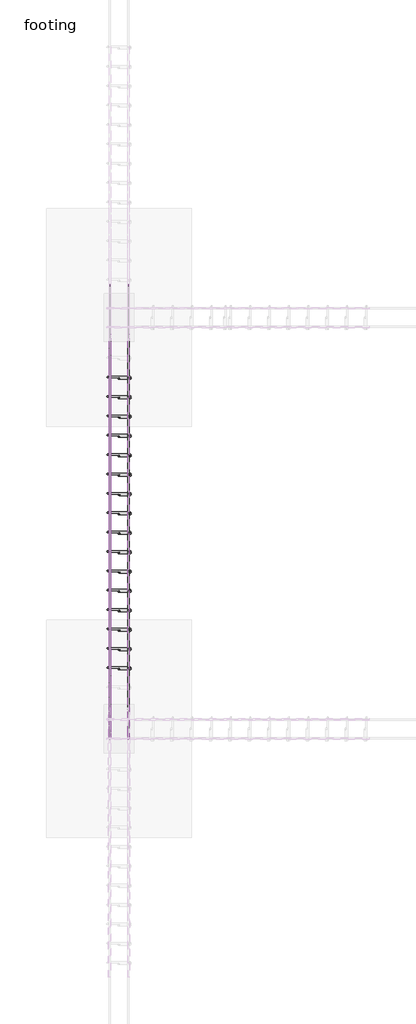
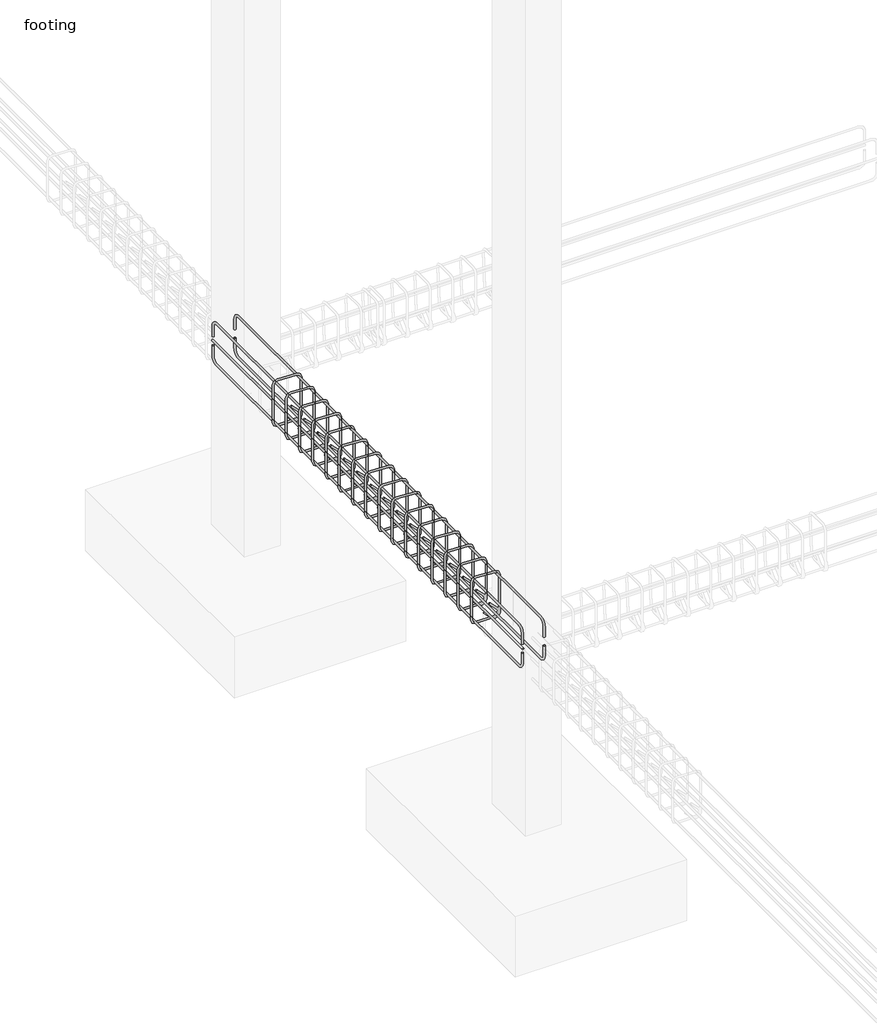
# One storey, part 5 of 21: 22 reinforcing bars.
"""IFC4 building model written with IfcOpenShell, lengths in millimetres."""

from ifc_helpers import new_model, si_unit, point, frame, origin, place, context, project, spatial, polyline, circle_curve, trimmed, segment, composite_curve, element, save
from ifc_brep_helpers import swept_disk

model = new_model("IFC4")

# Units and contexts
model_context = context("Model", 3, world=origin())
ifc_project = project(units=[si_unit("LENGTHUNIT", "METRE", prefix="MILLI")], contexts=[model_context])

# Site, building, storey
site = spatial("IfcSite", under=ifc_project)
building = spatial("IfcBuilding", under=site)
storey = spatial("IfcBuildingStorey", under=building, Name="footing", Elevation=-1524.0)

# Reinforcing bars
placement = place(None, origin())
element("IfcReinforcingBar", 1, at=placement, inside=storey, context=model_context, shape_type="SolidModel", body=[
    swept_disk(composite_curve([segment(polyline([(-12178.1165254, 4620.1956073, -265.9812362), (-12123.251527, 4620.1956073, -320.8462347)]), True, "CONTINUOUS"), segment(trimmed(circle_curve(frame((-12145.7021673, 4620.1956073, -343.296875), z_axis=(0.0, 1.0, 0.0), x_axis=(22.450640299999577, 0.0, 22.450640299999975)), 31.75), [point((-12123.251527, 4620.1956073, -320.8462347))], [point((-12145.7021673, 4620.1956073, -375.046875))], True, "CARTESIAN"), True, "CONTINUOUS"), segment(polyline([(-12145.7021673, 4620.1956073, -375.046875), (-12273.4959173, 4620.1956073, -375.046875)]), True, "CONTINUOUS"), segment(trimmed(circle_curve(frame((-12273.4959173, 4620.1956073, -343.296875), z_axis=(0.0, 1.0, 0.0), x_axis=(0.0, 0.0, -31.75)), 31.75), [point((-12273.4959173, 4620.1956073, -375.046875))], [point((-12305.2459173, 4620.1956073, -343.296875))], True, "CARTESIAN"), True, "CONTINUOUS"), segment(polyline([(-12305.2459173, 4620.1956073, -343.296875), (-12305.2459173, 4620.1956073, -63.103125)]), True, "CONTINUOUS"), segment(trimmed(circle_curve(frame((-12273.565658, 4618.0923536, -63.103125), z_axis=(0.0662442117686417, 0.9978034397651431, 0.0), x_axis=(-31.680259300001126, 2.1032537000000957, 0.0)), 31.75), [point((-12305.2459173, 4620.1956073, -63.103125))], [point((-12273.565658, 4618.0923536, -31.353125))], True, "CARTESIAN"), True, "CONTINUOUS"), segment(polyline([(-12273.565658, 4618.0923536, -31.353125), (-12145.6324265, 4609.598861, -31.353125)]), True, "CONTINUOUS"), segment(trimmed(circle_curve(frame((-12145.6324265, 4609.598861, -63.103125), z_axis=(0.06624421176864169, 0.997803439765143, 0.0), x_axis=(0.0, 0.0, 31.75)), 31.75), [point((-12145.6324265, 4609.598861, -31.353125))], [point((-12113.9521673, 4607.4956073, -63.103125))], True, "CARTESIAN"), True, "CONTINUOUS"), segment(polyline([(-12113.9521673, 4607.4956073, -63.103125), (-12113.9521673, 4607.4956073, -343.296875)]), True, "CONTINUOUS"), segment(trimmed(circle_curve(frame((-12145.7021673, 4607.4956073, -343.296875), z_axis=(0.0, 1.0, 0.0), x_axis=(31.75, 0.0, 0.0)), 31.75), [point((-12113.9521673, 4607.4956073, -343.296875))], [point((-12168.1528076, 4607.4956073, -365.7475153))], True, "CARTESIAN"), True, "CONTINUOUS"), segment(polyline([(-12168.1528076, 4607.4956073, -365.7475153), (-12223.017806, 4607.4956073, -310.8825168)]), True, "CONTINUOUS")], self_intersect=False), 6.35),
])
element("IfcReinforcingBar", 2, at=placement, inside=storey, context=model_context, shape_type="SolidModel", body=[
    swept_disk(composite_curve([segment(polyline([(-12178.1165254, 4782.8956073, -265.9812362), (-12123.251527, 4782.8956073, -320.8462347)]), True, "CONTINUOUS"), segment(trimmed(circle_curve(frame((-12145.7021673, 4782.8956073, -343.296875), z_axis=(0.0, 1.0, 0.0), x_axis=(22.450640299999577, 0.0, 22.450640299999975)), 31.75), [point((-12123.251527, 4782.8956073, -320.8462347))], [point((-12145.7021673, 4782.8956073, -375.046875))], True, "CARTESIAN"), True, "CONTINUOUS"), segment(polyline([(-12145.7021673, 4782.8956073, -375.046875), (-12273.4959173, 4782.8956073, -375.046875)]), True, "CONTINUOUS"), segment(trimmed(circle_curve(frame((-12273.4959173, 4782.8956073, -343.296875), z_axis=(0.0, 1.0, 0.0), x_axis=(0.0, 0.0, -31.75)), 31.75), [point((-12273.4959173, 4782.8956073, -375.046875))], [point((-12305.2459173, 4782.8956073, -343.296875))], True, "CARTESIAN"), True, "CONTINUOUS"), segment(polyline([(-12305.2459173, 4782.8956073, -343.296875), (-12305.2459173, 4782.8956073, -63.103125)]), True, "CONTINUOUS"), segment(trimmed(circle_curve(frame((-12273.565658, 4780.7923536, -63.103125), z_axis=(0.0662442117686417, 0.9978034397651431, 0.0), x_axis=(-31.680259300001126, 2.1032537000000957, 0.0)), 31.75), [point((-12305.2459173, 4782.8956073, -63.103125))], [point((-12273.565658, 4780.7923536, -31.353125))], True, "CARTESIAN"), True, "CONTINUOUS"), segment(polyline([(-12273.565658, 4780.7923536, -31.353125), (-12145.6324265, 4772.298861, -31.353125)]), True, "CONTINUOUS"), segment(trimmed(circle_curve(frame((-12145.6324265, 4772.298861, -63.103125), z_axis=(0.06624421176864169, 0.997803439765143, 0.0), x_axis=(0.0, 0.0, 31.75)), 31.75), [point((-12145.6324265, 4772.298861, -31.353125))], [point((-12113.9521673, 4770.1956073, -63.103125))], True, "CARTESIAN"), True, "CONTINUOUS"), segment(polyline([(-12113.9521673, 4770.1956073, -63.103125), (-12113.9521673, 4770.1956073, -343.296875)]), True, "CONTINUOUS"), segment(trimmed(circle_curve(frame((-12145.7021673, 4770.1956073, -343.296875), z_axis=(0.0, 1.0, 0.0), x_axis=(31.75, 0.0, 0.0)), 31.75), [point((-12113.9521673, 4770.1956073, -343.296875))], [point((-12168.1528076, 4770.1956073, -365.7475153))], True, "CARTESIAN"), True, "CONTINUOUS"), segment(polyline([(-12168.1528076, 4770.1956073, -365.7475153), (-12223.017806, 4770.1956073, -310.8825168)]), True, "CONTINUOUS")], self_intersect=False), 6.35),
])
element("IfcReinforcingBar", 3, at=placement, inside=storey, context=model_context, shape_type="SolidModel", body=[
    swept_disk(composite_curve([segment(polyline([(-12178.1165254, 4945.5956073, -265.9812362), (-12123.251527, 4945.5956073, -320.8462347)]), True, "CONTINUOUS"), segment(trimmed(circle_curve(frame((-12145.7021673, 4945.5956073, -343.296875), z_axis=(0.0, 1.0, 0.0), x_axis=(22.450640299999577, 0.0, 22.450640299999975)), 31.75), [point((-12123.251527, 4945.5956073, -320.8462347))], [point((-12145.7021673, 4945.5956073, -375.046875))], True, "CARTESIAN"), True, "CONTINUOUS"), segment(polyline([(-12145.7021673, 4945.5956073, -375.046875), (-12273.4959173, 4945.5956073, -375.046875)]), True, "CONTINUOUS"), segment(trimmed(circle_curve(frame((-12273.4959173, 4945.5956073, -343.296875), z_axis=(0.0, 1.0, 0.0), x_axis=(0.0, 0.0, -31.75)), 31.75), [point((-12273.4959173, 4945.5956073, -375.046875))], [point((-12305.2459173, 4945.5956073, -343.296875))], True, "CARTESIAN"), True, "CONTINUOUS"), segment(polyline([(-12305.2459173, 4945.5956073, -343.296875), (-12305.2459173, 4945.5956073, -63.103125)]), True, "CONTINUOUS"), segment(trimmed(circle_curve(frame((-12273.565658, 4943.4923536, -63.103125), z_axis=(0.0662442117686417, 0.9978034397651431, 0.0), x_axis=(-31.680259300001126, 2.1032537000000957, 0.0)), 31.75), [point((-12305.2459173, 4945.5956073, -63.103125))], [point((-12273.565658, 4943.4923536, -31.353125))], True, "CARTESIAN"), True, "CONTINUOUS"), segment(polyline([(-12273.565658, 4943.4923536, -31.353125), (-12145.6324265, 4934.998861, -31.353125)]), True, "CONTINUOUS"), segment(trimmed(circle_curve(frame((-12145.6324265, 4934.998861, -63.103125), z_axis=(0.06624421176864169, 0.997803439765143, 0.0), x_axis=(0.0, 0.0, 31.75)), 31.75), [point((-12145.6324265, 4934.998861, -31.353125))], [point((-12113.9521673, 4932.8956073, -63.103125))], True, "CARTESIAN"), True, "CONTINUOUS"), segment(polyline([(-12113.9521673, 4932.8956073, -63.103125), (-12113.9521673, 4932.8956073, -343.296875)]), True, "CONTINUOUS"), segment(trimmed(circle_curve(frame((-12145.7021673, 4932.8956073, -343.296875), z_axis=(0.0, 1.0, 0.0), x_axis=(31.75, 0.0, 0.0)), 31.75), [point((-12113.9521673, 4932.8956073, -343.296875))], [point((-12168.1528076, 4932.8956073, -365.7475153))], True, "CARTESIAN"), True, "CONTINUOUS"), segment(polyline([(-12168.1528076, 4932.8956073, -365.7475153), (-12223.017806, 4932.8956073, -310.8825168)]), True, "CONTINUOUS")], self_intersect=False), 6.35),
])
element("IfcReinforcingBar", 4, at=placement, inside=storey, context=model_context, shape_type="SolidModel", body=[
    swept_disk(composite_curve([segment(polyline([(-12178.1165254, 5108.2956073, -265.9812362), (-12123.251527, 5108.2956073, -320.8462347)]), True, "CONTINUOUS"), segment(trimmed(circle_curve(frame((-12145.7021673, 5108.2956073, -343.296875), z_axis=(0.0, 1.0, 0.0), x_axis=(22.450640299999577, 0.0, 22.450640299999975)), 31.75), [point((-12123.251527, 5108.2956073, -320.8462347))], [point((-12145.7021673, 5108.2956073, -375.046875))], True, "CARTESIAN"), True, "CONTINUOUS"), segment(polyline([(-12145.7021673, 5108.2956073, -375.046875), (-12273.4959173, 5108.2956073, -375.046875)]), True, "CONTINUOUS"), segment(trimmed(circle_curve(frame((-12273.4959173, 5108.2956073, -343.296875), z_axis=(0.0, 1.0, 0.0), x_axis=(0.0, 0.0, -31.75)), 31.75), [point((-12273.4959173, 5108.2956073, -375.046875))], [point((-12305.2459173, 5108.2956073, -343.296875))], True, "CARTESIAN"), True, "CONTINUOUS"), segment(polyline([(-12305.2459173, 5108.2956073, -343.296875), (-12305.2459173, 5108.2956073, -63.103125)]), True, "CONTINUOUS"), segment(trimmed(circle_curve(frame((-12273.565658, 5106.1923536, -63.103125), z_axis=(0.0662442117686417, 0.9978034397651431, 0.0), x_axis=(-31.680259300001126, 2.103253699999186, 0.0)), 31.75), [point((-12305.2459173, 5108.2956073, -63.103125))], [point((-12273.565658, 5106.1923536, -31.353125))], True, "CARTESIAN"), True, "CONTINUOUS"), segment(polyline([(-12273.565658, 5106.1923536, -31.353125), (-12145.6324265, 5097.698861, -31.353125)]), True, "CONTINUOUS"), segment(trimmed(circle_curve(frame((-12145.6324265, 5097.698861, -63.103125), z_axis=(0.06624421176864169, 0.997803439765143, 0.0), x_axis=(0.0, 0.0, 31.75)), 31.75), [point((-12145.6324265, 5097.698861, -31.353125))], [point((-12113.9521673, 5095.5956073, -63.103125))], True, "CARTESIAN"), True, "CONTINUOUS"), segment(polyline([(-12113.9521673, 5095.5956073, -63.103125), (-12113.9521673, 5095.5956073, -343.296875)]), True, "CONTINUOUS"), segment(trimmed(circle_curve(frame((-12145.7021673, 5095.5956073, -343.296875), z_axis=(0.0, 1.0, 0.0), x_axis=(31.75, 0.0, 0.0)), 31.75), [point((-12113.9521673, 5095.5956073, -343.296875))], [point((-12168.1528076, 5095.5956073, -365.7475153))], True, "CARTESIAN"), True, "CONTINUOUS"), segment(polyline([(-12168.1528076, 5095.5956073, -365.7475153), (-12223.017806, 5095.5956073, -310.8825168)]), True, "CONTINUOUS")], self_intersect=False), 6.35),
])
element("IfcReinforcingBar", 5, at=placement, inside=storey, context=model_context, shape_type="SolidModel", body=[
    swept_disk(composite_curve([segment(polyline([(-12178.1165254, 5270.9956073, -265.9812362), (-12123.251527, 5270.9956073, -320.8462347)]), True, "CONTINUOUS"), segment(trimmed(circle_curve(frame((-12145.7021673, 5270.9956073, -343.296875), z_axis=(0.0, 1.0, 0.0), x_axis=(22.450640299999577, 0.0, 22.450640299999975)), 31.75), [point((-12123.251527, 5270.9956073, -320.8462347))], [point((-12145.7021673, 5270.9956073, -375.046875))], True, "CARTESIAN"), True, "CONTINUOUS"), segment(polyline([(-12145.7021673, 5270.9956073, -375.046875), (-12273.4959173, 5270.9956073, -375.046875)]), True, "CONTINUOUS"), segment(trimmed(circle_curve(frame((-12273.4959173, 5270.9956073, -343.296875), z_axis=(0.0, 1.0, 0.0), x_axis=(0.0, 0.0, -31.75)), 31.75), [point((-12273.4959173, 5270.9956073, -375.046875))], [point((-12305.2459173, 5270.9956073, -343.296875))], True, "CARTESIAN"), True, "CONTINUOUS"), segment(polyline([(-12305.2459173, 5270.9956073, -343.296875), (-12305.2459173, 5270.9956073, -63.103125)]), True, "CONTINUOUS"), segment(trimmed(circle_curve(frame((-12273.565658, 5268.8923536, -63.103125), z_axis=(0.0662442117686417, 0.9978034397651431, 0.0), x_axis=(-31.680259300001126, 2.1032537000000957, 0.0)), 31.75), [point((-12305.2459173, 5270.9956073, -63.103125))], [point((-12273.565658, 5268.8923536, -31.353125))], True, "CARTESIAN"), True, "CONTINUOUS"), segment(polyline([(-12273.565658, 5268.8923536, -31.353125), (-12145.6324265, 5260.398861, -31.353125)]), True, "CONTINUOUS"), segment(trimmed(circle_curve(frame((-12145.6324265, 5260.398861, -63.103125), z_axis=(0.06624421176864169, 0.997803439765143, 0.0), x_axis=(0.0, 0.0, 31.75)), 31.75), [point((-12145.6324265, 5260.398861, -31.353125))], [point((-12113.9521673, 5258.2956073, -63.103125))], True, "CARTESIAN"), True, "CONTINUOUS"), segment(polyline([(-12113.9521673, 5258.2956073, -63.103125), (-12113.9521673, 5258.2956073, -343.296875)]), True, "CONTINUOUS"), segment(trimmed(circle_curve(frame((-12145.7021673, 5258.2956073, -343.296875), z_axis=(0.0, 1.0, 0.0), x_axis=(31.75, 0.0, 0.0)), 31.75), [point((-12113.9521673, 5258.2956073, -343.296875))], [point((-12168.1528076, 5258.2956073, -365.7475153))], True, "CARTESIAN"), True, "CONTINUOUS"), segment(polyline([(-12168.1528076, 5258.2956073, -365.7475153), (-12223.017806, 5258.2956073, -310.8825168)]), True, "CONTINUOUS")], self_intersect=False), 6.35),
])
element("IfcReinforcingBar", 6, at=placement, inside=storey, context=model_context, shape_type="SolidModel", body=[
    swept_disk(composite_curve([segment(polyline([(-12178.1165254, 5433.6956073, -265.9812362), (-12123.251527, 5433.6956073, -320.8462347)]), True, "CONTINUOUS"), segment(trimmed(circle_curve(frame((-12145.7021673, 5433.6956073, -343.296875), z_axis=(0.0, 1.0, 0.0), x_axis=(22.450640299999577, 0.0, 22.450640299999975)), 31.75), [point((-12123.251527, 5433.6956073, -320.8462347))], [point((-12145.7021673, 5433.6956073, -375.046875))], True, "CARTESIAN"), True, "CONTINUOUS"), segment(polyline([(-12145.7021673, 5433.6956073, -375.046875), (-12273.4959173, 5433.6956073, -375.046875)]), True, "CONTINUOUS"), segment(trimmed(circle_curve(frame((-12273.4959173, 5433.6956073, -343.296875), z_axis=(0.0, 1.0, 0.0), x_axis=(0.0, 0.0, -31.75)), 31.75), [point((-12273.4959173, 5433.6956073, -375.046875))], [point((-12305.2459173, 5433.6956073, -343.296875))], True, "CARTESIAN"), True, "CONTINUOUS"), segment(polyline([(-12305.2459173, 5433.6956073, -343.296875), (-12305.2459173, 5433.6956073, -63.103125)]), True, "CONTINUOUS"), segment(trimmed(circle_curve(frame((-12273.565658, 5431.5923536, -63.103125), z_axis=(0.0662442117686417, 0.9978034397651431, 0.0), x_axis=(-31.680259300001126, 2.1032537000000957, 0.0)), 31.75), [point((-12305.2459173, 5433.6956073, -63.103125))], [point((-12273.565658, 5431.5923536, -31.353125))], True, "CARTESIAN"), True, "CONTINUOUS"), segment(polyline([(-12273.565658, 5431.5923536, -31.353125), (-12145.6324265, 5423.098861, -31.353125)]), True, "CONTINUOUS"), segment(trimmed(circle_curve(frame((-12145.6324265, 5423.098861, -63.103125), z_axis=(0.06624421176864169, 0.997803439765143, 0.0), x_axis=(0.0, 0.0, 31.75)), 31.75), [point((-12145.6324265, 5423.098861, -31.353125))], [point((-12113.9521673, 5420.9956073, -63.103125))], True, "CARTESIAN"), True, "CONTINUOUS"), segment(polyline([(-12113.9521673, 5420.9956073, -63.103125), (-12113.9521673, 5420.9956073, -343.296875)]), True, "CONTINUOUS"), segment(trimmed(circle_curve(frame((-12145.7021673, 5420.9956073, -343.296875), z_axis=(0.0, 1.0, 0.0), x_axis=(31.75, 0.0, 0.0)), 31.75), [point((-12113.9521673, 5420.9956073, -343.296875))], [point((-12168.1528076, 5420.9956073, -365.7475153))], True, "CARTESIAN"), True, "CONTINUOUS"), segment(polyline([(-12168.1528076, 5420.9956073, -365.7475153), (-12223.017806, 5420.9956073, -310.8825168)]), True, "CONTINUOUS")], self_intersect=False), 6.35),
])
element("IfcReinforcingBar", 7, at=placement, inside=storey, context=model_context, shape_type="SolidModel", body=[
    swept_disk(composite_curve([segment(polyline([(-12178.1165254, 5596.3956073, -265.9812362), (-12123.251527, 5596.3956073, -320.8462347)]), True, "CONTINUOUS"), segment(trimmed(circle_curve(frame((-12145.7021673, 5596.3956073, -343.296875), z_axis=(0.0, 1.0, 0.0), x_axis=(22.450640299999577, 0.0, 22.450640299999975)), 31.75), [point((-12123.251527, 5596.3956073, -320.8462347))], [point((-12145.7021673, 5596.3956073, -375.046875))], True, "CARTESIAN"), True, "CONTINUOUS"), segment(polyline([(-12145.7021673, 5596.3956073, -375.046875), (-12273.4959173, 5596.3956073, -375.046875)]), True, "CONTINUOUS"), segment(trimmed(circle_curve(frame((-12273.4959173, 5596.3956073, -343.296875), z_axis=(0.0, 1.0, 0.0), x_axis=(0.0, 0.0, -31.75)), 31.75), [point((-12273.4959173, 5596.3956073, -375.046875))], [point((-12305.2459173, 5596.3956073, -343.296875))], True, "CARTESIAN"), True, "CONTINUOUS"), segment(polyline([(-12305.2459173, 5596.3956073, -343.296875), (-12305.2459173, 5596.3956073, -63.103125)]), True, "CONTINUOUS"), segment(trimmed(circle_curve(frame((-12273.565658, 5594.2923536, -63.103125), z_axis=(0.0662442117686417, 0.9978034397651431, 0.0), x_axis=(-31.680259300001126, 2.1032537000000957, 0.0)), 31.75), [point((-12305.2459173, 5596.3956073, -63.103125))], [point((-12273.565658, 5594.2923536, -31.353125))], True, "CARTESIAN"), True, "CONTINUOUS"), segment(polyline([(-12273.565658, 5594.2923536, -31.353125), (-12145.6324265, 5585.798861, -31.353125)]), True, "CONTINUOUS"), segment(trimmed(circle_curve(frame((-12145.6324265, 5585.798861, -63.103125), z_axis=(0.06624421176864169, 0.997803439765143, 0.0), x_axis=(0.0, 0.0, 31.75)), 31.75), [point((-12145.6324265, 5585.798861, -31.353125))], [point((-12113.9521673, 5583.6956073, -63.103125))], True, "CARTESIAN"), True, "CONTINUOUS"), segment(polyline([(-12113.9521673, 5583.6956073, -63.103125), (-12113.9521673, 5583.6956073, -343.296875)]), True, "CONTINUOUS"), segment(trimmed(circle_curve(frame((-12145.7021673, 5583.6956073, -343.296875), z_axis=(0.0, 1.0, 0.0), x_axis=(31.75, 0.0, 0.0)), 31.75), [point((-12113.9521673, 5583.6956073, -343.296875))], [point((-12168.1528076, 5583.6956073, -365.7475153))], True, "CARTESIAN"), True, "CONTINUOUS"), segment(polyline([(-12168.1528076, 5583.6956073, -365.7475153), (-12223.017806, 5583.6956073, -310.8825168)]), True, "CONTINUOUS")], self_intersect=False), 6.35),
])
element("IfcReinforcingBar", 8, at=placement, inside=storey, context=model_context, shape_type="SolidModel", body=[
    swept_disk(composite_curve([segment(polyline([(-12178.1165254, 5759.0956073, -265.9812362), (-12123.251527, 5759.0956073, -320.8462347)]), True, "CONTINUOUS"), segment(trimmed(circle_curve(frame((-12145.7021673, 5759.0956073, -343.296875), z_axis=(0.0, 1.0, 0.0), x_axis=(22.450640299999577, 0.0, 22.450640299999975)), 31.75), [point((-12123.251527, 5759.0956073, -320.8462347))], [point((-12145.7021673, 5759.0956073, -375.046875))], True, "CARTESIAN"), True, "CONTINUOUS"), segment(polyline([(-12145.7021673, 5759.0956073, -375.046875), (-12273.4959173, 5759.0956073, -375.046875)]), True, "CONTINUOUS"), segment(trimmed(circle_curve(frame((-12273.4959173, 5759.0956073, -343.296875), z_axis=(0.0, 1.0, 0.0), x_axis=(0.0, 0.0, -31.75)), 31.75), [point((-12273.4959173, 5759.0956073, -375.046875))], [point((-12305.2459173, 5759.0956073, -343.296875))], True, "CARTESIAN"), True, "CONTINUOUS"), segment(polyline([(-12305.2459173, 5759.0956073, -343.296875), (-12305.2459173, 5759.0956073, -63.103125)]), True, "CONTINUOUS"), segment(trimmed(circle_curve(frame((-12273.565658, 5756.9923536, -63.103125), z_axis=(0.0662442117686417, 0.9978034397651431, 0.0), x_axis=(-31.680259300001126, 2.1032537000000957, 0.0)), 31.75), [point((-12305.2459173, 5759.0956073, -63.103125))], [point((-12273.565658, 5756.9923536, -31.353125))], True, "CARTESIAN"), True, "CONTINUOUS"), segment(polyline([(-12273.565658, 5756.9923536, -31.353125), (-12145.6324265, 5748.498861, -31.353125)]), True, "CONTINUOUS"), segment(trimmed(circle_curve(frame((-12145.6324265, 5748.498861, -63.103125), z_axis=(0.06624421176864169, 0.997803439765143, 0.0), x_axis=(0.0, 0.0, 31.75)), 31.75), [point((-12145.6324265, 5748.498861, -31.353125))], [point((-12113.9521673, 5746.3956073, -63.103125))], True, "CARTESIAN"), True, "CONTINUOUS"), segment(polyline([(-12113.9521673, 5746.3956073, -63.103125), (-12113.9521673, 5746.3956073, -343.296875)]), True, "CONTINUOUS"), segment(trimmed(circle_curve(frame((-12145.7021673, 5746.3956073, -343.296875), z_axis=(0.0, 1.0, 0.0), x_axis=(31.75, 0.0, 0.0)), 31.75), [point((-12113.9521673, 5746.3956073, -343.296875))], [point((-12168.1528076, 5746.3956073, -365.7475153))], True, "CARTESIAN"), True, "CONTINUOUS"), segment(polyline([(-12168.1528076, 5746.3956073, -365.7475153), (-12223.017806, 5746.3956073, -310.8825168)]), True, "CONTINUOUS")], self_intersect=False), 6.35),
])
element("IfcReinforcingBar", 9, at=placement, inside=storey, context=model_context, shape_type="SolidModel", body=[
    swept_disk(composite_curve([segment(polyline([(-12178.1165254, 5921.7956073, -265.9812362), (-12123.251527, 5921.7956073, -320.8462347)]), True, "CONTINUOUS"), segment(trimmed(circle_curve(frame((-12145.7021673, 5921.7956073, -343.296875), z_axis=(0.0, 1.0, 0.0), x_axis=(22.450640299999577, 0.0, 22.450640299999975)), 31.75), [point((-12123.251527, 5921.7956073, -320.8462347))], [point((-12145.7021673, 5921.7956073, -375.046875))], True, "CARTESIAN"), True, "CONTINUOUS"), segment(polyline([(-12145.7021673, 5921.7956073, -375.046875), (-12273.4959173, 5921.7956073, -375.046875)]), True, "CONTINUOUS"), segment(trimmed(circle_curve(frame((-12273.4959173, 5921.7956073, -343.296875), z_axis=(0.0, 1.0, 0.0), x_axis=(0.0, 0.0, -31.75)), 31.75), [point((-12273.4959173, 5921.7956073, -375.046875))], [point((-12305.2459173, 5921.7956073, -343.296875))], True, "CARTESIAN"), True, "CONTINUOUS"), segment(polyline([(-12305.2459173, 5921.7956073, -343.296875), (-12305.2459173, 5921.7956073, -63.103125)]), True, "CONTINUOUS"), segment(trimmed(circle_curve(frame((-12273.565658, 5919.6923536, -63.103125), z_axis=(0.0662442117686417, 0.9978034397651431, 0.0), x_axis=(-31.680259300001126, 2.103253699999186, 0.0)), 31.75), [point((-12305.2459173, 5921.7956073, -63.103125))], [point((-12273.565658, 5919.6923536, -31.353125))], True, "CARTESIAN"), True, "CONTINUOUS"), segment(polyline([(-12273.565658, 5919.6923536, -31.353125), (-12145.6324265, 5911.198861, -31.353125)]), True, "CONTINUOUS"), segment(trimmed(circle_curve(frame((-12145.6324265, 5911.198861, -63.103125), z_axis=(0.06624421176864169, 0.997803439765143, 0.0), x_axis=(0.0, 0.0, 31.75)), 31.75), [point((-12145.6324265, 5911.198861, -31.353125))], [point((-12113.9521673, 5909.0956073, -63.103125))], True, "CARTESIAN"), True, "CONTINUOUS"), segment(polyline([(-12113.9521673, 5909.0956073, -63.103125), (-12113.9521673, 5909.0956073, -343.296875)]), True, "CONTINUOUS"), segment(trimmed(circle_curve(frame((-12145.7021673, 5909.0956073, -343.296875), z_axis=(0.0, 1.0, 0.0), x_axis=(31.75, 0.0, 0.0)), 31.75), [point((-12113.9521673, 5909.0956073, -343.296875))], [point((-12168.1528076, 5909.0956073, -365.7475153))], True, "CARTESIAN"), True, "CONTINUOUS"), segment(polyline([(-12168.1528076, 5909.0956073, -365.7475153), (-12223.017806, 5909.0956073, -310.8825168)]), True, "CONTINUOUS")], self_intersect=False), 6.35),
])
element("IfcReinforcingBar", 10, at=placement, inside=storey, context=model_context, shape_type="SolidModel", body=[
    swept_disk(composite_curve([segment(polyline([(-12178.1165254, 6084.4956073, -265.9812362), (-12123.251527, 6084.4956073, -320.8462347)]), True, "CONTINUOUS"), segment(trimmed(circle_curve(frame((-12145.7021673, 6084.4956073, -343.296875), z_axis=(0.0, 1.0, 0.0), x_axis=(22.450640299999577, 0.0, 22.450640299999975)), 31.75), [point((-12123.251527, 6084.4956073, -320.8462347))], [point((-12145.7021673, 6084.4956073, -375.046875))], True, "CARTESIAN"), True, "CONTINUOUS"), segment(polyline([(-12145.7021673, 6084.4956073, -375.046875), (-12273.4959173, 6084.4956073, -375.046875)]), True, "CONTINUOUS"), segment(trimmed(circle_curve(frame((-12273.4959173, 6084.4956073, -343.296875), z_axis=(0.0, 1.0, 0.0), x_axis=(0.0, 0.0, -31.75)), 31.75), [point((-12273.4959173, 6084.4956073, -375.046875))], [point((-12305.2459173, 6084.4956073, -343.296875))], True, "CARTESIAN"), True, "CONTINUOUS"), segment(polyline([(-12305.2459173, 6084.4956073, -343.296875), (-12305.2459173, 6084.4956073, -63.103125)]), True, "CONTINUOUS"), segment(trimmed(circle_curve(frame((-12273.565658, 6082.3923536, -63.103125), z_axis=(0.0662442117686417, 0.9978034397651431, 0.0), x_axis=(-31.680259300001126, 2.1032537000000957, 0.0)), 31.75), [point((-12305.2459173, 6084.4956073, -63.103125))], [point((-12273.565658, 6082.3923536, -31.353125))], True, "CARTESIAN"), True, "CONTINUOUS"), segment(polyline([(-12273.565658, 6082.3923536, -31.353125), (-12145.6324265, 6073.898861, -31.353125)]), True, "CONTINUOUS"), segment(trimmed(circle_curve(frame((-12145.6324265, 6073.898861, -63.103125), z_axis=(0.06624421176864169, 0.997803439765143, 0.0), x_axis=(0.0, 0.0, 31.75)), 31.75), [point((-12145.6324265, 6073.898861, -31.353125))], [point((-12113.9521673, 6071.7956073, -63.103125))], True, "CARTESIAN"), True, "CONTINUOUS"), segment(polyline([(-12113.9521673, 6071.7956073, -63.103125), (-12113.9521673, 6071.7956073, -343.296875)]), True, "CONTINUOUS"), segment(trimmed(circle_curve(frame((-12145.7021673, 6071.7956073, -343.296875), z_axis=(0.0, 1.0, 0.0), x_axis=(31.75, 0.0, 0.0)), 31.75), [point((-12113.9521673, 6071.7956073, -343.296875))], [point((-12168.1528076, 6071.7956073, -365.7475153))], True, "CARTESIAN"), True, "CONTINUOUS"), segment(polyline([(-12168.1528076, 6071.7956073, -365.7475153), (-12223.017806, 6071.7956073, -310.8825168)]), True, "CONTINUOUS")], self_intersect=False), 6.35),
])
element("IfcReinforcingBar", 11, at=placement, inside=storey, context=model_context, shape_type="SolidModel", body=[
    swept_disk(composite_curve([segment(polyline([(-12178.1165254, 6247.1956073, -265.9812362), (-12123.251527, 6247.1956073, -320.8462347)]), True, "CONTINUOUS"), segment(trimmed(circle_curve(frame((-12145.7021673, 6247.1956073, -343.296875), z_axis=(0.0, 1.0, 0.0), x_axis=(22.450640299999577, 0.0, 22.450640299999975)), 31.75), [point((-12123.251527, 6247.1956073, -320.8462347))], [point((-12145.7021673, 6247.1956073, -375.046875))], True, "CARTESIAN"), True, "CONTINUOUS"), segment(polyline([(-12145.7021673, 6247.1956073, -375.046875), (-12273.4959173, 6247.1956073, -375.046875)]), True, "CONTINUOUS"), segment(trimmed(circle_curve(frame((-12273.4959173, 6247.1956073, -343.296875), z_axis=(0.0, 1.0, 0.0), x_axis=(0.0, 0.0, -31.75)), 31.75), [point((-12273.4959173, 6247.1956073, -375.046875))], [point((-12305.2459173, 6247.1956073, -343.296875))], True, "CARTESIAN"), True, "CONTINUOUS"), segment(polyline([(-12305.2459173, 6247.1956073, -343.296875), (-12305.2459173, 6247.1956073, -63.103125)]), True, "CONTINUOUS"), segment(trimmed(circle_curve(frame((-12273.565658, 6245.0923536, -63.103125), z_axis=(0.0662442117686417, 0.9978034397651431, 0.0), x_axis=(-31.680259300001126, 2.1032537000000957, 0.0)), 31.75), [point((-12305.2459173, 6247.1956073, -63.103125))], [point((-12273.565658, 6245.0923536, -31.353125))], True, "CARTESIAN"), True, "CONTINUOUS"), segment(polyline([(-12273.565658, 6245.0923536, -31.353125), (-12145.6324265, 6236.598861, -31.353125)]), True, "CONTINUOUS"), segment(trimmed(circle_curve(frame((-12145.6324265, 6236.598861, -63.103125), z_axis=(0.06624421176864169, 0.997803439765143, 0.0), x_axis=(0.0, 0.0, 31.75)), 31.75), [point((-12145.6324265, 6236.598861, -31.353125))], [point((-12113.9521673, 6234.4956073, -63.103125))], True, "CARTESIAN"), True, "CONTINUOUS"), segment(polyline([(-12113.9521673, 6234.4956073, -63.103125), (-12113.9521673, 6234.4956073, -343.296875)]), True, "CONTINUOUS"), segment(trimmed(circle_curve(frame((-12145.7021673, 6234.4956073, -343.296875), z_axis=(0.0, 1.0, 0.0), x_axis=(31.75, 0.0, 0.0)), 31.75), [point((-12113.9521673, 6234.4956073, -343.296875))], [point((-12168.1528076, 6234.4956073, -365.7475153))], True, "CARTESIAN"), True, "CONTINUOUS"), segment(polyline([(-12168.1528076, 6234.4956073, -365.7475153), (-12223.017806, 6234.4956073, -310.8825168)]), True, "CONTINUOUS")], self_intersect=False), 6.35),
])
element("IfcReinforcingBar", 12, at=placement, inside=storey, context=model_context, shape_type="SolidModel", body=[
    swept_disk(composite_curve([segment(polyline([(-12178.1165254, 6409.8956073, -265.9812362), (-12123.251527, 6409.8956073, -320.8462347)]), True, "CONTINUOUS"), segment(trimmed(circle_curve(frame((-12145.7021673, 6409.8956073, -343.296875), z_axis=(0.0, 1.0, 0.0), x_axis=(22.450640299999577, 0.0, 22.450640299999975)), 31.75), [point((-12123.251527, 6409.8956073, -320.8462347))], [point((-12145.7021673, 6409.8956073, -375.046875))], True, "CARTESIAN"), True, "CONTINUOUS"), segment(polyline([(-12145.7021673, 6409.8956073, -375.046875), (-12273.4959173, 6409.8956073, -375.046875)]), True, "CONTINUOUS"), segment(trimmed(circle_curve(frame((-12273.4959173, 6409.8956073, -343.296875), z_axis=(0.0, 1.0, 0.0), x_axis=(0.0, 0.0, -31.75)), 31.75), [point((-12273.4959173, 6409.8956073, -375.046875))], [point((-12305.2459173, 6409.8956073, -343.296875))], True, "CARTESIAN"), True, "CONTINUOUS"), segment(polyline([(-12305.2459173, 6409.8956073, -343.296875), (-12305.2459173, 6409.8956073, -63.103125)]), True, "CONTINUOUS"), segment(trimmed(circle_curve(frame((-12273.565658, 6407.7923536, -63.103125), z_axis=(0.0662442117686417, 0.9978034397651431, 0.0), x_axis=(-31.680259300001126, 2.1032537000000957, 0.0)), 31.75), [point((-12305.2459173, 6409.8956073, -63.103125))], [point((-12273.565658, 6407.7923536, -31.353125))], True, "CARTESIAN"), True, "CONTINUOUS"), segment(polyline([(-12273.565658, 6407.7923536, -31.353125), (-12145.6324265, 6399.298861, -31.353125)]), True, "CONTINUOUS"), segment(trimmed(circle_curve(frame((-12145.6324265, 6399.298861, -63.103125), z_axis=(0.06624421176864169, 0.997803439765143, 0.0), x_axis=(0.0, 0.0, 31.75)), 31.75), [point((-12145.6324265, 6399.298861, -31.353125))], [point((-12113.9521673, 6397.1956073, -63.103125))], True, "CARTESIAN"), True, "CONTINUOUS"), segment(polyline([(-12113.9521673, 6397.1956073, -63.103125), (-12113.9521673, 6397.1956073, -343.296875)]), True, "CONTINUOUS"), segment(trimmed(circle_curve(frame((-12145.7021673, 6397.1956073, -343.296875), z_axis=(0.0, 1.0, 0.0), x_axis=(31.75, 0.0, 0.0)), 31.75), [point((-12113.9521673, 6397.1956073, -343.296875))], [point((-12168.1528076, 6397.1956073, -365.7475153))], True, "CARTESIAN"), True, "CONTINUOUS"), segment(polyline([(-12168.1528076, 6397.1956073, -365.7475153), (-12223.017806, 6397.1956073, -310.8825168)]), True, "CONTINUOUS")], self_intersect=False), 6.35),
])
element("IfcReinforcingBar", 13, at=placement, inside=storey, context=model_context, shape_type="SolidModel", body=[
    swept_disk(composite_curve([segment(polyline([(-12178.1165254, 6572.5956073, -265.9812362), (-12123.251527, 6572.5956073, -320.8462347)]), True, "CONTINUOUS"), segment(trimmed(circle_curve(frame((-12145.7021673, 6572.5956073, -343.296875), z_axis=(0.0, 1.0, 0.0), x_axis=(22.450640299999577, 0.0, 22.450640299999975)), 31.75), [point((-12123.251527, 6572.5956073, -320.8462347))], [point((-12145.7021673, 6572.5956073, -375.046875))], True, "CARTESIAN"), True, "CONTINUOUS"), segment(polyline([(-12145.7021673, 6572.5956073, -375.046875), (-12273.4959173, 6572.5956073, -375.046875)]), True, "CONTINUOUS"), segment(trimmed(circle_curve(frame((-12273.4959173, 6572.5956073, -343.296875), z_axis=(0.0, 1.0, 0.0), x_axis=(0.0, 0.0, -31.75)), 31.75), [point((-12273.4959173, 6572.5956073, -375.046875))], [point((-12305.2459173, 6572.5956073, -343.296875))], True, "CARTESIAN"), True, "CONTINUOUS"), segment(polyline([(-12305.2459173, 6572.5956073, -343.296875), (-12305.2459173, 6572.5956073, -63.103125)]), True, "CONTINUOUS"), segment(trimmed(circle_curve(frame((-12273.565658, 6570.4923536, -63.103125), z_axis=(0.0662442117686417, 0.9978034397651431, 0.0), x_axis=(-31.680259300001126, 2.1032537000000957, 0.0)), 31.75), [point((-12305.2459173, 6572.5956073, -63.103125))], [point((-12273.565658, 6570.4923536, -31.353125))], True, "CARTESIAN"), True, "CONTINUOUS"), segment(polyline([(-12273.565658, 6570.4923536, -31.353125), (-12145.6324265, 6561.998861, -31.353125)]), True, "CONTINUOUS"), segment(trimmed(circle_curve(frame((-12145.6324265, 6561.998861, -63.103125), z_axis=(0.06624421176864169, 0.997803439765143, 0.0), x_axis=(0.0, 0.0, 31.75)), 31.75), [point((-12145.6324265, 6561.998861, -31.353125))], [point((-12113.9521673, 6559.8956073, -63.103125))], True, "CARTESIAN"), True, "CONTINUOUS"), segment(polyline([(-12113.9521673, 6559.8956073, -63.103125), (-12113.9521673, 6559.8956073, -343.296875)]), True, "CONTINUOUS"), segment(trimmed(circle_curve(frame((-12145.7021673, 6559.8956073, -343.296875), z_axis=(0.0, 1.0, 0.0), x_axis=(31.75, 0.0, 0.0)), 31.75), [point((-12113.9521673, 6559.8956073, -343.296875))], [point((-12168.1528076, 6559.8956073, -365.7475153))], True, "CARTESIAN"), True, "CONTINUOUS"), segment(polyline([(-12168.1528076, 6559.8956073, -365.7475153), (-12223.017806, 6559.8956073, -310.8825168)]), True, "CONTINUOUS")], self_intersect=False), 6.35),
])
element("IfcReinforcingBar", 14, at=placement, inside=storey, context=model_context, shape_type="SolidModel", body=[
    swept_disk(composite_curve([segment(polyline([(-12178.1165254, 6735.2956073, -265.9812362), (-12123.251527, 6735.2956073, -320.8462347)]), True, "CONTINUOUS"), segment(trimmed(circle_curve(frame((-12145.7021673, 6735.2956073, -343.296875), z_axis=(0.0, 1.0, 0.0), x_axis=(22.450640299999577, 0.0, 22.450640299999975)), 31.75), [point((-12123.251527, 6735.2956073, -320.8462347))], [point((-12145.7021673, 6735.2956073, -375.046875))], True, "CARTESIAN"), True, "CONTINUOUS"), segment(polyline([(-12145.7021673, 6735.2956073, -375.046875), (-12273.4959173, 6735.2956073, -375.046875)]), True, "CONTINUOUS"), segment(trimmed(circle_curve(frame((-12273.4959173, 6735.2956073, -343.296875), z_axis=(0.0, 1.0, 0.0), x_axis=(0.0, 0.0, -31.75)), 31.75), [point((-12273.4959173, 6735.2956073, -375.046875))], [point((-12305.2459173, 6735.2956073, -343.296875))], True, "CARTESIAN"), True, "CONTINUOUS"), segment(polyline([(-12305.2459173, 6735.2956073, -343.296875), (-12305.2459173, 6735.2956073, -63.103125)]), True, "CONTINUOUS"), segment(trimmed(circle_curve(frame((-12273.565658, 6733.1923536, -63.103125), z_axis=(0.0662442117686417, 0.9978034397651431, 0.0), x_axis=(-31.680259300001126, 2.103253699999186, 0.0)), 31.75), [point((-12305.2459173, 6735.2956073, -63.103125))], [point((-12273.565658, 6733.1923536, -31.353125))], True, "CARTESIAN"), True, "CONTINUOUS"), segment(polyline([(-12273.565658, 6733.1923536, -31.353125), (-12145.6324265, 6724.698861, -31.353125)]), True, "CONTINUOUS"), segment(trimmed(circle_curve(frame((-12145.6324265, 6724.698861, -63.103125), z_axis=(0.06624421176864169, 0.997803439765143, 0.0), x_axis=(0.0, 0.0, 31.75)), 31.75), [point((-12145.6324265, 6724.698861, -31.353125))], [point((-12113.9521673, 6722.5956073, -63.103125))], True, "CARTESIAN"), True, "CONTINUOUS"), segment(polyline([(-12113.9521673, 6722.5956073, -63.103125), (-12113.9521673, 6722.5956073, -343.296875)]), True, "CONTINUOUS"), segment(trimmed(circle_curve(frame((-12145.7021673, 6722.5956073, -343.296875), z_axis=(0.0, 1.0, 0.0), x_axis=(31.75, 0.0, 0.0)), 31.75), [point((-12113.9521673, 6722.5956073, -343.296875))], [point((-12168.1528076, 6722.5956073, -365.7475153))], True, "CARTESIAN"), True, "CONTINUOUS"), segment(polyline([(-12168.1528076, 6722.5956073, -365.7475153), (-12223.017806, 6722.5956073, -310.8825168)]), True, "CONTINUOUS")], self_intersect=False), 6.35),
])
element("IfcReinforcingBar", 15, at=placement, inside=storey, context=model_context, shape_type="SolidModel", body=[
    swept_disk(composite_curve([segment(polyline([(-12178.1165254, 6897.9956073, -265.9812362), (-12123.251527, 6897.9956073, -320.8462347)]), True, "CONTINUOUS"), segment(trimmed(circle_curve(frame((-12145.7021673, 6897.9956073, -343.296875), z_axis=(0.0, 1.0, 0.0), x_axis=(22.450640299999577, 0.0, 22.450640299999975)), 31.75), [point((-12123.251527, 6897.9956073, -320.8462347))], [point((-12145.7021673, 6897.9956073, -375.046875))], True, "CARTESIAN"), True, "CONTINUOUS"), segment(polyline([(-12145.7021673, 6897.9956073, -375.046875), (-12273.4959173, 6897.9956073, -375.046875)]), True, "CONTINUOUS"), segment(trimmed(circle_curve(frame((-12273.4959173, 6897.9956073, -343.296875), z_axis=(0.0, 1.0, 0.0), x_axis=(0.0, 0.0, -31.75)), 31.75), [point((-12273.4959173, 6897.9956073, -375.046875))], [point((-12305.2459173, 6897.9956073, -343.296875))], True, "CARTESIAN"), True, "CONTINUOUS"), segment(polyline([(-12305.2459173, 6897.9956073, -343.296875), (-12305.2459173, 6897.9956073, -63.103125)]), True, "CONTINUOUS"), segment(trimmed(circle_curve(frame((-12273.565658, 6895.8923536, -63.103125), z_axis=(0.0662442117686417, 0.9978034397651431, 0.0), x_axis=(-31.680259300001126, 2.1032537000000957, 0.0)), 31.75), [point((-12305.2459173, 6897.9956073, -63.103125))], [point((-12273.565658, 6895.8923536, -31.353125))], True, "CARTESIAN"), True, "CONTINUOUS"), segment(polyline([(-12273.565658, 6895.8923536, -31.353125), (-12145.6324265, 6887.398861, -31.353125)]), True, "CONTINUOUS"), segment(trimmed(circle_curve(frame((-12145.6324265, 6887.398861, -63.103125), z_axis=(0.06624421176864169, 0.997803439765143, 0.0), x_axis=(0.0, 0.0, 31.75)), 31.75), [point((-12145.6324265, 6887.398861, -31.353125))], [point((-12113.9521673, 6885.2956073, -63.103125))], True, "CARTESIAN"), True, "CONTINUOUS"), segment(polyline([(-12113.9521673, 6885.2956073, -63.103125), (-12113.9521673, 6885.2956073, -343.296875)]), True, "CONTINUOUS"), segment(trimmed(circle_curve(frame((-12145.7021673, 6885.2956073, -343.296875), z_axis=(0.0, 1.0, 0.0), x_axis=(31.75, 0.0, 0.0)), 31.75), [point((-12113.9521673, 6885.2956073, -343.296875))], [point((-12168.1528076, 6885.2956073, -365.7475153))], True, "CARTESIAN"), True, "CONTINUOUS"), segment(polyline([(-12168.1528076, 6885.2956073, -365.7475153), (-12223.017806, 6885.2956073, -310.8825168)]), True, "CONTINUOUS")], self_intersect=False), 6.35),
])
element("IfcReinforcingBar", 16, at=placement, inside=storey, context=model_context, shape_type="SolidModel", body=[
    swept_disk(composite_curve([segment(polyline([(-12178.1165254, 7060.6956073, -265.9812362), (-12123.251527, 7060.6956073, -320.8462347)]), True, "CONTINUOUS"), segment(trimmed(circle_curve(frame((-12145.7021673, 7060.6956073, -343.296875), z_axis=(0.0, 1.0, 0.0), x_axis=(22.450640299999577, 0.0, 22.450640299999975)), 31.75), [point((-12123.251527, 7060.6956073, -320.8462347))], [point((-12145.7021673, 7060.6956073, -375.046875))], True, "CARTESIAN"), True, "CONTINUOUS"), segment(polyline([(-12145.7021673, 7060.6956073, -375.046875), (-12273.4959173, 7060.6956073, -375.046875)]), True, "CONTINUOUS"), segment(trimmed(circle_curve(frame((-12273.4959173, 7060.6956073, -343.296875), z_axis=(0.0, 1.0, 0.0), x_axis=(0.0, 0.0, -31.75)), 31.75), [point((-12273.4959173, 7060.6956073, -375.046875))], [point((-12305.2459173, 7060.6956073, -343.296875))], True, "CARTESIAN"), True, "CONTINUOUS"), segment(polyline([(-12305.2459173, 7060.6956073, -343.296875), (-12305.2459173, 7060.6956073, -63.103125)]), True, "CONTINUOUS"), segment(trimmed(circle_curve(frame((-12273.565658, 7058.5923536, -63.103125), z_axis=(0.0662442117686417, 0.9978034397651431, 0.0), x_axis=(-31.680259300001126, 2.1032537000000957, 0.0)), 31.75), [point((-12305.2459173, 7060.6956073, -63.103125))], [point((-12273.565658, 7058.5923536, -31.353125))], True, "CARTESIAN"), True, "CONTINUOUS"), segment(polyline([(-12273.565658, 7058.5923536, -31.353125), (-12145.6324265, 7050.098861, -31.353125)]), True, "CONTINUOUS"), segment(trimmed(circle_curve(frame((-12145.6324265, 7050.098861, -63.103125), z_axis=(0.06624421176864169, 0.997803439765143, 0.0), x_axis=(0.0, 0.0, 31.75)), 31.75), [point((-12145.6324265, 7050.098861, -31.353125))], [point((-12113.9521673, 7047.9956073, -63.103125))], True, "CARTESIAN"), True, "CONTINUOUS"), segment(polyline([(-12113.9521673, 7047.9956073, -63.103125), (-12113.9521673, 7047.9956073, -343.296875)]), True, "CONTINUOUS"), segment(trimmed(circle_curve(frame((-12145.7021673, 7047.9956073, -343.296875), z_axis=(0.0, 1.0, 0.0), x_axis=(31.75, 0.0, 0.0)), 31.75), [point((-12113.9521673, 7047.9956073, -343.296875))], [point((-12168.1528076, 7047.9956073, -365.7475153))], True, "CARTESIAN"), True, "CONTINUOUS"), segment(polyline([(-12168.1528076, 7047.9956073, -365.7475153), (-12223.017806, 7047.9956073, -310.8825168)]), True, "CONTINUOUS")], self_intersect=False), 6.35),
])
element("IfcReinforcingBar", 17, at=placement, inside=storey, context=model_context, shape_type="SolidModel", body=[
    swept_disk(composite_curve([segment(polyline([(-12132.2317831, 4024.7359344, -170.2827408), (-12132.2317831, 4024.7359344, -94.0827408)]), True, "CONTINUOUS"), segment(trimmed(circle_curve(frame((-12132.2317831, 4069.1859344, -94.0827408), z_axis=(-1.0, 0.0, 0.0), x_axis=(0.0, -44.44999999999982, 0.0)), 44.45), [point((-12132.2317831, 4024.7359344, -94.0827408))], [point((-12132.2317831, 4069.1859344, -49.6327408))], True, "CARTESIAN"), True, "CONTINUOUS"), segment(polyline([(-12132.2317831, 4069.1859344, -49.6327408), (-12132.2317831, 7786.2668244, -49.6327408)]), True, "CONTINUOUS"), segment(trimmed(circle_curve(frame((-12132.2317831, 7786.2668244, -94.0827408), z_axis=(-1.0, 0.0, 0.0), x_axis=(0.0, 0.0, 44.449999999999996)), 44.45), [point((-12132.2317831, 7786.2668244, -49.6327408))], [point((-12132.2317831, 7830.7168244, -94.0827408))], True, "CARTESIAN"), True, "CONTINUOUS"), segment(polyline([(-12132.2317831, 7830.7168244, -94.0827408), (-12132.2317831, 7830.7168244, -170.2827408)]), True, "CONTINUOUS")], self_intersect=False), 6.35),
])
element("IfcReinforcingBar", 18, at=placement, inside=storey, context=model_context, shape_type="SolidModel", body=[
    swept_disk(composite_curve([segment(polyline([(-12286.9663014, 4024.7359344, -170.2827408), (-12286.9663014, 4024.7359344, -94.0827408)]), True, "CONTINUOUS"), segment(trimmed(circle_curve(frame((-12286.9663014, 4069.1859344, -94.0827408), z_axis=(-1.0, 0.0, 0.0), x_axis=(0.0, -44.44999999999982, 0.0)), 44.45), [point((-12286.9663014, 4024.7359344, -94.0827408))], [point((-12286.9663014, 4069.1859344, -49.6327408))], True, "CARTESIAN"), True, "CONTINUOUS"), segment(polyline([(-12286.9663014, 4069.1859344, -49.6327408), (-12286.9663014, 7786.2668244, -49.6327408)]), True, "CONTINUOUS"), segment(trimmed(circle_curve(frame((-12286.9663014, 7786.2668244, -94.0827408), z_axis=(-1.0, 0.0, 0.0), x_axis=(0.0, 0.0, 44.449999999999996)), 44.45), [point((-12286.9663014, 7786.2668244, -49.6327408))], [point((-12286.9663014, 7830.7168244, -94.0827408))], True, "CARTESIAN"), True, "CONTINUOUS"), segment(polyline([(-12286.9663014, 7830.7168244, -94.0827408), (-12286.9663014, 7830.7168244, -170.2827408)]), True, "CONTINUOUS")], self_intersect=False), 6.35),
])
element("IfcReinforcingBar", 19, at=placement, inside=storey, context=model_context, shape_type="SolidModel", body=[
    swept_disk(composite_curve([segment(polyline([(-12132.2317831, 4024.7359344, -236.1172592), (-12132.2317831, 4024.7359344, -312.3172592)]), True, "CONTINUOUS"), segment(trimmed(circle_curve(frame((-12132.2317831, 4069.1859344, -312.3172592), z_axis=(1.0, 0.0, 0.0), x_axis=(0.0, -44.44999999999982, 0.0)), 44.45), [point((-12132.2317831, 4024.7359344, -312.3172592))], [point((-12132.2317831, 4069.1859344, -356.7672592))], True, "CARTESIAN"), True, "CONTINUOUS"), segment(polyline([(-12132.2317831, 4069.1859344, -356.7672592), (-12132.2317831, 7786.2668244, -356.7672592)]), True, "CONTINUOUS"), segment(trimmed(circle_curve(frame((-12132.2317831, 7786.2668244, -312.3172592), z_axis=(1.0, 0.0, 0.0), x_axis=(0.0, 0.0, -44.44999999999999)), 44.45), [point((-12132.2317831, 7786.2668244, -356.7672592))], [point((-12132.2317831, 7830.7168244, -312.3172592))], True, "CARTESIAN"), True, "CONTINUOUS"), segment(polyline([(-12132.2317831, 7830.7168244, -312.3172592), (-12132.2317831, 7830.7168244, -236.1172592)]), True, "CONTINUOUS")], self_intersect=False), 6.35),
])
element("IfcReinforcingBar", 20, at=placement, inside=storey, context=model_context, shape_type="SolidModel", body=[
    swept_disk(composite_curve([segment(polyline([(-12286.9663014, 4024.7359344, -236.1172592), (-12286.9663014, 4024.7359344, -312.3172592)]), True, "CONTINUOUS"), segment(trimmed(circle_curve(frame((-12286.9663014, 4069.1859344, -312.3172592), z_axis=(1.0, 0.0, 0.0), x_axis=(0.0, -44.44999999999982, 0.0)), 44.45), [point((-12286.9663014, 4024.7359344, -312.3172592))], [point((-12286.9663014, 4069.1859344, -356.7672592))], True, "CARTESIAN"), True, "CONTINUOUS"), segment(polyline([(-12286.9663014, 4069.1859344, -356.7672592), (-12286.9663014, 7786.2668244, -356.7672592)]), True, "CONTINUOUS"), segment(trimmed(circle_curve(frame((-12286.9663014, 7786.2668244, -312.3172592), z_axis=(1.0, 0.0, 0.0), x_axis=(0.0, 0.0, -44.44999999999999)), 44.45), [point((-12286.9663014, 7786.2668244, -356.7672592))], [point((-12286.9663014, 7830.7168244, -312.3172592))], True, "CARTESIAN"), True, "CONTINUOUS"), segment(polyline([(-12286.9663014, 7830.7168244, -312.3172592), (-12286.9663014, 7830.7168244, -236.1172592)]), True, "CONTINUOUS")], self_intersect=False), 6.35),
])
element("IfcReinforcingBar", 21, at=placement, inside=storey, context=model_context, shape_type="SolidModel", body=[
    swept_disk(composite_curve([segment(polyline([(-12286.9663014, 4018.3859344, -203.2), (-12286.9663014, 7837.0668244, -203.2)]), True, "CONTINUOUS")], self_intersect=False), 6.35),
])
element("IfcReinforcingBar", 22, at=placement, inside=storey, context=model_context, shape_type="SolidModel", body=[
    swept_disk(composite_curve([segment(polyline([(-12286.9663014, 4018.3859344, -203.2), (-12286.9663014, 7837.0668244, -203.2)]), True, "CONTINUOUS")], self_intersect=False), 6.35),
])

save(model, "model.ifc")

# Revit data of these elements
# Elements 1, 2, 3, 4, 5, 6, 7, 8, 9, 10, 11, 12, 13, 14, 15, 16, 17, 18, 19, 20, 21, 22 (IfcReinforcingBar)
#   Phase Created = New Construction
